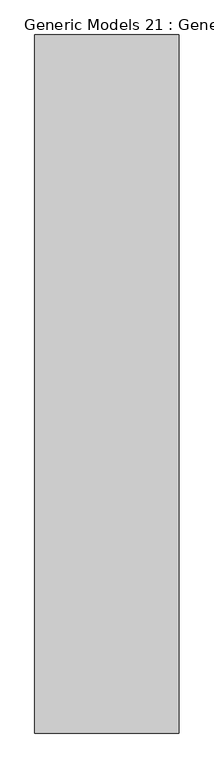
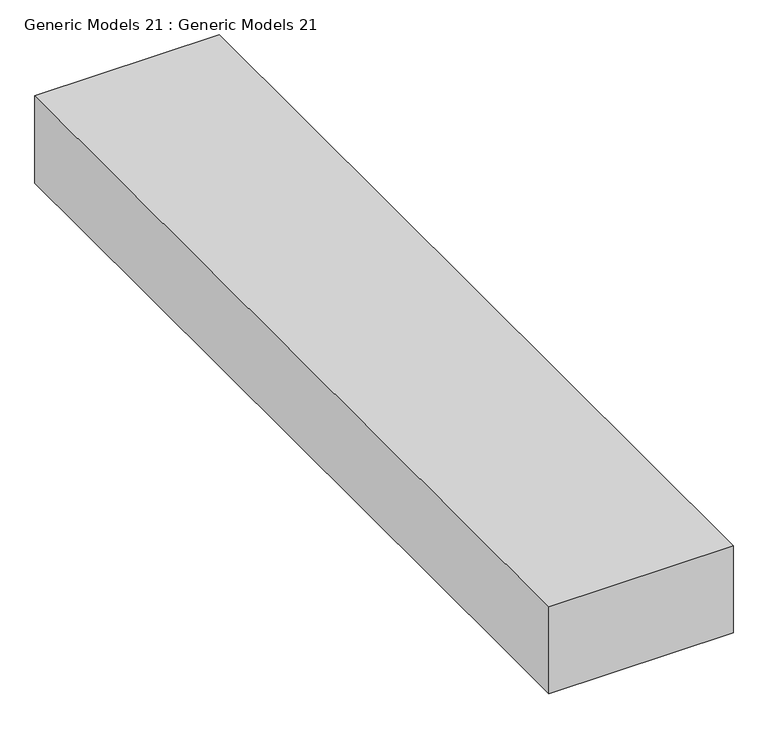
"""IFC4 building model written with IfcOpenShell, lengths in millimetres: proxy geometry, Generic Models 21 : Generic Models 21."""

from ifc_helpers import new_model, si_unit, frame, origin, place, context, project, spatial, polyline, outline, extrude, source, transform, mapped, element, save


def generic_models_21_generic_models_21_87948dc1(model_context):
    return source(origin(), model_context, "Body", "SweptSolid", [
        extrude(outline(polyline([(-844.8190997, 17459.2), (-2064.0190997, 17459.2), (-2191.0190997, 17459.2), (-2191.0190997, 17611.6), (-717.8190997, 17611.6), (-717.8190997, 17459.2), (-844.8190997, 17459.2)])), frame((4567.1987798, 0.0, 0.0), z_axis=(1.0, 0.0, 0.0), x_axis=(0.0, 1.0, 0.0)), (0.0, 0.0, 1.0), 304.8),
    ])


if __name__ == "__main__":
    model = new_model("IFC4")
    model_context = context("Model", 3, world=origin())
    ifc_project = project(units=[si_unit("LENGTHUNIT", "METRE", prefix="MILLI")], contexts=[model_context])
    site = spatial("IfcSite", under=ifc_project)
    building = spatial("IfcBuilding", under=site)
    placement = place(None, origin())
    generic_models_21_generic_models_21_shape = generic_models_21_generic_models_21_87948dc1(model_context)
    element("IfcBuildingElementProxy", 1, Name="Generic Models 21 : Generic Models 21", ObjectType="Generic Models 21 : Generic Models 21", at=placement, inside=building, context=model_context, shape_type="MappedRepresentation", body=[
        mapped(generic_models_21_generic_models_21_shape, transform((0.0, 0.0, 0.0), x_axis=(1.0, 0.0, 0.0), y_axis=(0.0, 1.0, 0.0), z_axis=(0.0, 0.0, 1.0))),
    ])
    save(model, "model.ifc")

# Revit data of these elements
# Element 1 (IfcBuildingElementProxy, "Generic Models 21 : Generic Models 21")
#   Materials on its faces: "white"
# Materials
#   "white": class "Generic", colour RGB 120 120 120, transparency 0, Cost = 0
